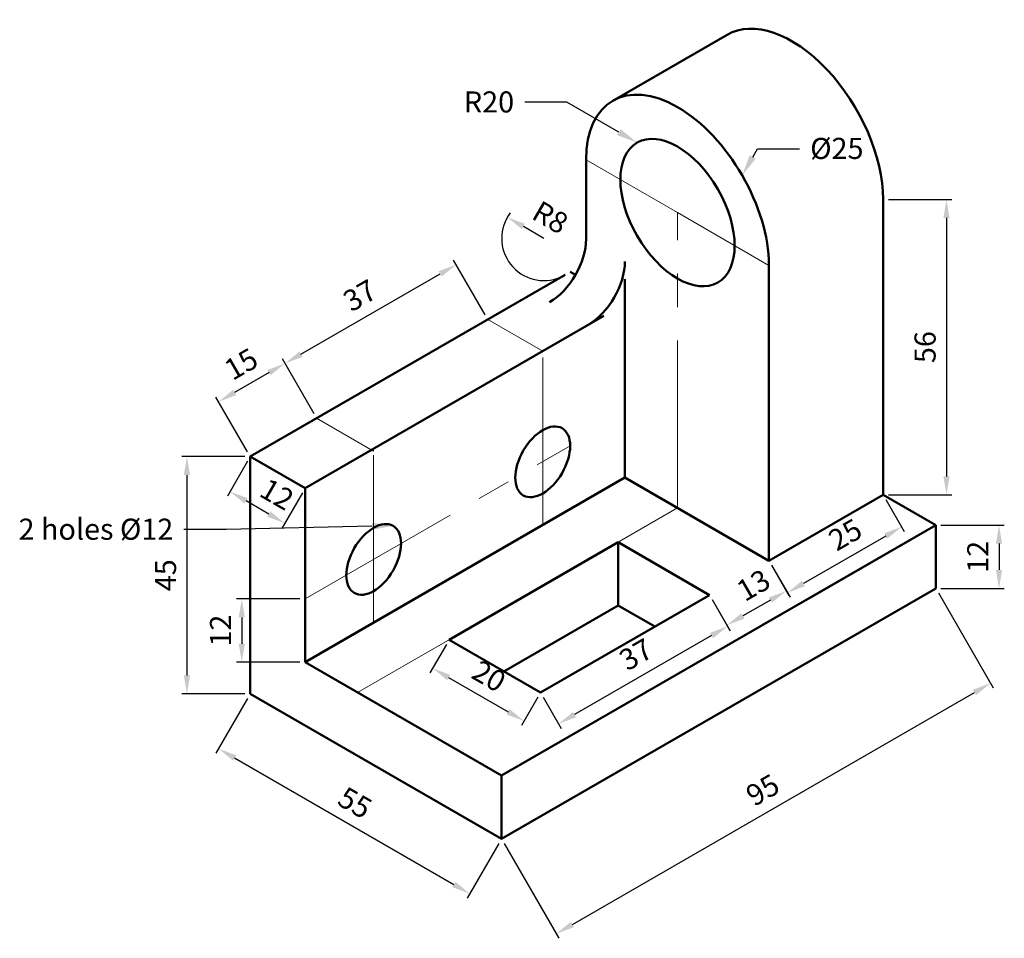
# Model space of a CAD drawing. Units: millimetres. Extents: x 1729 to 1916, y 2075 to 2249.
import ezdxf
from ezdxf import colors
from ezdxf.entities.mleader import LeaderData, LeaderLine
from ezdxf.math import Vec2, Vec3

# ---------------------------------------------------------------- set-up
doc = ezdxf.new("R2010")
doc.units = ezdxf.units.MM
doc.linetypes.add('CENTER', pattern=[50.8, 31.75, -6.35, 6.35, -6.35])
for name, color, linetype, lineweight in [('M-CNTR', 4, 'CENTER', 18), ('M-DIMS', 3, 'Continuous', 25), ('M-OUTL', 7, 'Continuous', 50)]:
    doc.layers.add(name, color=color, linetype=linetype, lineweight=lineweight)
doc.styles.get("Standard").update_dxf_attribs({"font": 'arial.ttf'})
doc.dimstyles.new('AM_ISO$0', dxfattribs={"dimtxt": 4, "dimasz": 3.5, "dimexe": 1, "dimexo": 1, "dimgap": 1.5, "dimtad": 1, "dimdsep": 46, "dimtxsty": 'Standard', "dimcen": 0, "dimclrd": 256, "dimclre": 256, "dimclrt": 2, "dimadec": 0, "dimazin": 2, "dimtp": 0.1, "dimtm": 0.1, "dimtfac": 0.71, "dimtmove": 0, "dimatfit": 3, "dimfxl": 1, "dimlwd": -1, "dimlwe": -1, "dimarcsym": 1})
doc.dimstyles.new('AM_ISO$4', dxfattribs={"dimtxt": 4, "dimasz": 3.5, "dimexe": 1, "dimexo": 1, "dimgap": 1.5, "dimtad": 1, "dimtoh": 1, "dimdsep": 46, "dimtxsty": 'Standard', "dimcen": 0, "dimclrd": 256, "dimclre": 256, "dimclrt": 2, "dimadec": 0, "dimazin": 2, "dimtp": 0.1, "dimtm": 0.1, "dimtfac": 0.71, "dimtofl": 0, "dimtmove": 0, "dimatfit": 0, "dimfxl": 1, "dimlwd": -1, "dimlwe": -1, "dimarcsym": 1})

# ---------------------------------------------------------------- blocks, each defined once
blk = doc.blocks.new('*D3')
at = {"layer": 'Defpoints', "color": 0, "transparency": 16777216}
for p in [(1902.52, 2141.34), (1912.9, 2123.37), (1820.25, 2093.84)]:
    blk.add_point(p, dxfattribs=at)
at = {"layer": 'M-DIMS', "color": 0, "linetype": 'ByBlock', "transparency": 16777216}
for p, q in [((1903.02, 2140.48), (1913.4, 2122.51)), ((1833.66, 2077.62), (1909.87, 2121.62)), ((1820.75, 2092.98), (1831.12, 2075.01))]:
    blk.add_line(p, q, dxfattribs=at)
at = {"layer": 'M-DIMS', "color": 0, "transparency": 16777216}
for points in [[(1909.57, 2122.13), (1910.16, 2121.12), (1912.9, 2123.37)], [(1833.36, 2078.13), (1833.95, 2077.12), (1830.62, 2075.87)]]:
    blk.add_solid(points, dxfattribs=at)
at = {"layer": 'M-DIMS', "color": 0, "transparency": 16777216, "insert": (1869.99, 2102.69), "char_height": 4, "attachment_point": 5, "rotation": 30}
blk.add_mtext('95', dxfattribs=at)
blk = doc.blocks.new('*D4')
at = {"layer": 'Defpoints', "color": 0, "transparency": 16777216}
for p in [(1902.52, 2153.34), (1902.52, 2141.34), (1914.52, 2141.34)]:
    blk.add_point(p, dxfattribs=at)
at = {"layer": 'M-DIMS', "color": 0, "linetype": 'ByBlock', "transparency": 16777216}
for p, q in [((1903.52, 2153.34), (1915.52, 2153.34)), ((1914.52, 2149.84), (1914.52, 2144.84)), ((1903.52, 2141.34), (1915.52, 2141.34))]:
    blk.add_line(p, q, dxfattribs=at)
at = {"layer": 'M-DIMS', "color": 0, "transparency": 16777216}
for points in [[(1913.94, 2149.84), (1915.1, 2149.84), (1914.52, 2153.34)], [(1913.94, 2144.84), (1915.1, 2144.84), (1914.52, 2141.34)]]:
    blk.add_solid(points, dxfattribs=at)
at = {"layer": 'M-DIMS', "color": 0, "transparency": 16777216, "insert": (1911.01, 2147.34), "char_height": 4, "attachment_point": 5, "rotation": 90}
blk.add_mtext('12', dxfattribs=at)
blk = doc.blocks.new('*D5')
at = {"layer": 'Defpoints', "color": 0, "transparency": 16777216}
for p in [(1892.56, 2159.09), (1870.91, 2146.59), (1874.42, 2140.52)]:
    blk.add_point(p, dxfattribs=at)
at = {"layer": 'M-DIMS', "color": 0, "linetype": 'ByBlock', "transparency": 16777216}
for p, q in [((1893.06, 2158.23), (1896.57, 2152.16)), ((1893.04, 2151.27), (1877.45, 2142.27)), ((1871.41, 2145.73), (1874.92, 2139.66))]:
    blk.add_line(p, q, dxfattribs=at)
at = {"layer": 'M-DIMS', "color": 0, "transparency": 16777216}
for points in [[(1892.74, 2151.78), (1893.33, 2150.77), (1896.07, 2153.02)], [(1877.16, 2142.78), (1877.74, 2141.77), (1874.42, 2140.52)]]:
    blk.add_solid(points, dxfattribs=at)
at = {"layer": 'M-DIMS', "color": 0, "transparency": 16777216, "insert": (1885.63, 2151.09), "char_height": 4, "attachment_point": 5, "rotation": 30}
blk.add_mtext('25', dxfattribs=at)
blk = doc.blocks.new('*D6')
at = {"layer": 'Defpoints', "color": 0, "transparency": 16777216}
for p in [(1772.62, 2166.34), (1768.78, 2159.7), (1783.01, 2160.34)]:
    blk.add_point(p, dxfattribs=at)
at = {"layer": 'M-DIMS', "color": 0, "linetype": 'ByBlock', "transparency": 16777216}
for p, q in [((1772.12, 2165.48), (1768.28, 2158.83)), ((1782.51, 2159.48), (1778.67, 2152.83)), ((1776.14, 2155.45), (1771.81, 2157.95))]:
    blk.add_line(p, q, dxfattribs=at)
at = {"layer": 'M-DIMS', "color": 0, "transparency": 16777216}
for points in [[(1772.1, 2158.45), (1771.52, 2157.44), (1768.78, 2159.7)], [(1776.43, 2155.95), (1775.85, 2154.94), (1779.17, 2153.7)]]:
    blk.add_solid(points, dxfattribs=at)
at = {"layer": 'M-DIMS', "color": 0, "transparency": 16777216, "insert": (1777.43, 2158.75), "char_height": 4, "attachment_point": 5, "rotation": 330}
blk.add_mtext('12', dxfattribs=at)
blk = doc.blocks.new('*D7')
at = {"layer": 'Defpoints', "color": 0, "transparency": 16777216}
for p in [(1772.62, 2166.34), (1760.62, 2121.34), (1772.62, 2121.34)]:
    blk.add_point(p, dxfattribs=at)
at = {"layer": 'M-DIMS', "color": 0, "linetype": 'ByBlock', "transparency": 16777216}
for p, q in [((1771.62, 2166.34), (1759.62, 2166.34)), ((1760.62, 2162.84), (1760.62, 2124.84)), ((1771.62, 2121.34), (1759.62, 2121.34))]:
    blk.add_line(p, q, dxfattribs=at)
at = {"layer": 'M-DIMS', "color": 0, "transparency": 16777216}
for points in [[(1760.03, 2162.84), (1761.2, 2162.84), (1760.62, 2166.34)], [(1760.03, 2124.84), (1761.2, 2124.84), (1760.62, 2121.34)]]:
    blk.add_solid(points, dxfattribs=at)
at = {"layer": 'M-DIMS', "color": 0, "transparency": 16777216, "insert": (1757.08, 2143.84), "char_height": 4, "attachment_point": 5, "rotation": 90}
blk.add_mtext('45', dxfattribs=at)
blk = doc.blocks.new('*D8')
at = {"layer": 'Defpoints', "color": 0, "transparency": 16777216}
for p in [(1892.56, 2215.09), (1892.56, 2159.09), (1904.56, 2159.09)]:
    blk.add_point(p, dxfattribs=at)
at = {"layer": 'M-DIMS', "color": 0, "linetype": 'ByBlock', "transparency": 16777216}
for p, q in [((1893.56, 2215.09), (1905.56, 2215.09)), ((1904.56, 2211.59), (1904.56, 2162.59)), ((1893.56, 2159.09), (1905.56, 2159.09))]:
    blk.add_line(p, q, dxfattribs=at)
at = {"layer": 'M-DIMS', "color": 0, "transparency": 16777216}
for points in [[(1903.98, 2211.59), (1905.14, 2211.59), (1904.56, 2215.09)], [(1903.98, 2162.59), (1905.14, 2162.59), (1904.56, 2159.09)]]:
    blk.add_solid(points, dxfattribs=at)
at = {"layer": 'M-DIMS', "color": 0, "transparency": 16777216, "insert": (1901.02, 2187.09), "char_height": 4, "attachment_point": 5, "rotation": 90}
blk.add_mtext('56', dxfattribs=at)
blk = doc.blocks.new('*D9')
at = {"layer": 'Defpoints', "color": 0, "transparency": 16777216}
for p in [(1870.91, 2146.59), (1859.65, 2140.09), (1862.95, 2134.37)]:
    blk.add_point(p, dxfattribs=at)
at = {"layer": 'M-DIMS', "color": 0, "linetype": 'ByBlock', "transparency": 16777216}
for p, q in [((1871.41, 2145.73), (1874.71, 2140.01)), ((1860.15, 2139.23), (1863.45, 2133.51)), ((1871.18, 2139.12), (1865.99, 2136.12))]:
    blk.add_line(p, q, dxfattribs=at)
at = {"layer": 'M-DIMS', "color": 0, "transparency": 16777216}
for points in [[(1870.89, 2139.63), (1871.47, 2138.62), (1874.21, 2140.87)], [(1865.69, 2136.63), (1866.28, 2135.62), (1862.95, 2134.37)]]:
    blk.add_solid(points, dxfattribs=at)
at = {"layer": 'M-DIMS', "color": 0, "transparency": 16777216, "insert": (1868.24, 2141.52), "char_height": 4, "attachment_point": 5, "rotation": 30}
blk.add_mtext('13', dxfattribs=at)
blk = doc.blocks.new('*D10')
at = {"layer": 'Defpoints', "color": 0, "transparency": 16777216}
for p in [(1859.65, 2140.09), (1827.61, 2121.59), (1831.03, 2115.66)]:
    blk.add_point(p, dxfattribs=at)
at = {"layer": 'M-DIMS', "color": 0, "linetype": 'ByBlock', "transparency": 16777216}
for p, q in [((1860.15, 2139.23), (1863.58, 2133.29)), ((1860.05, 2132.41), (1834.07, 2117.41)), ((1828.11, 2120.73), (1831.53, 2114.79))]:
    blk.add_line(p, q, dxfattribs=at)
at = {"layer": 'M-DIMS', "color": 0, "transparency": 16777216}
for points in [[(1859.75, 2132.92), (1860.34, 2131.91), (1863.08, 2134.16)], [(1833.77, 2117.92), (1834.36, 2116.91), (1831.03, 2115.66)]]:
    blk.add_solid(points, dxfattribs=at)
at = {"layer": 'M-DIMS', "color": 0, "transparency": 16777216, "insert": (1845.96, 2128.37), "char_height": 4, "attachment_point": 5, "rotation": 30}
blk.add_mtext('37', dxfattribs=at)
blk = doc.blocks.new('*D11')
at = {"layer": 'Defpoints', "color": 0, "transparency": 16777216}
for p in [(1810.29, 2131.59), (1827.61, 2121.59), (1824.5, 2116.21)]:
    blk.add_point(p, dxfattribs=at)
at = {"layer": 'M-DIMS', "color": 0, "linetype": 'ByBlock', "transparency": 16777216}
for p, q in [((1809.79, 2130.73), (1806.68, 2125.34)), ((1810.21, 2124.46), (1821.47, 2117.96)), ((1827.11, 2120.73), (1824, 2115.34))]:
    blk.add_line(p, q, dxfattribs=at)
at = {"layer": 'M-DIMS', "color": 0, "transparency": 16777216}
for points in [[(1810.5, 2124.96), (1809.92, 2123.95), (1807.18, 2126.21)], [(1821.76, 2118.46), (1821.18, 2117.45), (1824.5, 2116.21)]]:
    blk.add_solid(points, dxfattribs=at)
at = {"layer": 'M-DIMS', "color": 0, "transparency": 16777216, "insert": (1817.61, 2124.27), "char_height": 4, "attachment_point": 5, "rotation": 330}
blk.add_mtext('20', dxfattribs=at)
blk = doc.blocks.new('*D12')
at = {"layer": 'Defpoints', "color": 0, "transparency": 16777216}
for p in [(1772.62, 2121.34), (1820.25, 2093.84), (1814.25, 2083.45)]:
    blk.add_point(p, dxfattribs=at)
at = {"layer": 'M-DIMS', "color": 0, "linetype": 'ByBlock', "transparency": 16777216}
for p, q in [((1772.12, 2120.48), (1766.12, 2110.09)), ((1769.65, 2109.2), (1811.22, 2085.2)), ((1819.75, 2092.98), (1813.75, 2082.59))]:
    blk.add_line(p, q, dxfattribs=at)
at = {"layer": 'M-DIMS', "color": 0, "transparency": 16777216}
for points in [[(1769.94, 2109.71), (1769.36, 2108.7), (1766.62, 2110.95)], [(1811.51, 2085.71), (1810.92, 2084.7), (1814.25, 2083.45)]]:
    blk.add_solid(points, dxfattribs=at)
at = {"layer": 'M-DIMS', "color": 0, "transparency": 16777216, "insert": (1792.2, 2100.26), "char_height": 4, "attachment_point": 5, "rotation": 330}
blk.add_mtext('55', dxfattribs=at)
blk = doc.blocks.new('*D13')
at = {"layer": 'Defpoints', "color": 0, "transparency": 16777216}
for p in [(1811.65, 2202.74), (1817.65, 2192.34), (1785.2, 2173.61)]:
    blk.add_point(p, dxfattribs=at)
at = {"layer": 'M-DIMS', "color": 0, "linetype": 'ByBlock', "transparency": 16777216}
for p, q in [((1817.15, 2193.21), (1811.15, 2203.6)), ((1782.23, 2185.75), (1808.62, 2200.99)), ((1784.7, 2174.47), (1778.7, 2184.87))]:
    blk.add_line(p, q, dxfattribs=at)
at = {"layer": 'M-DIMS', "color": 0, "transparency": 16777216}
for points in [[(1808.33, 2201.49), (1808.91, 2200.48), (1811.65, 2202.74)], [(1781.94, 2186.25), (1782.52, 2185.24), (1779.2, 2184)]]:
    blk.add_solid(points, dxfattribs=at)
at = {"layer": 'M-DIMS', "color": 0, "transparency": 16777216, "insert": (1793.65, 2196.44), "char_height": 4, "attachment_point": 5, "rotation": 30}
blk.add_mtext('37', dxfattribs=at)
blk = doc.blocks.new('*D14')
at = {"layer": 'Defpoints', "color": 0, "transparency": 16777216}
for p in [(1766.62, 2176.74), (1785.2, 2173.61), (1772.62, 2166.34)]:
    blk.add_point(p, dxfattribs=at)
at = {"layer": 'M-DIMS', "color": 0, "linetype": 'ByBlock', "transparency": 16777216}
for p, q in [((1784.7, 2174.47), (1778.7, 2184.87)), ((1776.17, 2182.25), (1769.65, 2178.49)), ((1772.12, 2167.21), (1766.12, 2177.6))]:
    blk.add_line(p, q, dxfattribs=at)
at = {"layer": 'M-DIMS', "color": 0, "transparency": 16777216}
for points in [[(1775.87, 2182.75), (1776.46, 2181.74), (1779.2, 2184)], [(1769.36, 2178.99), (1769.94, 2177.98), (1766.62, 2176.74)]]:
    blk.add_solid(points, dxfattribs=at)
at = {"layer": 'M-DIMS', "color": 0, "transparency": 16777216, "insert": (1771.14, 2183.44), "char_height": 4, "attachment_point": 5, "rotation": 30}
blk.add_mtext('15', dxfattribs=at)
blk = doc.blocks.new('*D15')
at = {"layer": 'Defpoints', "color": 0, "transparency": 16777216}
for p in [(1821.34, 2211.71), (1828.27, 2207.71)]:
    blk.add_point(p, dxfattribs=at)
at = {"layer": 'M-DIMS', "color": 0, "linetype": 'ByBlock', "transparency": 16777216}
blk.add_line((1828.27, 2207.71), (1824.37, 2209.96), dxfattribs=at)
blk.add_arc((1828.27, 2207.71), 8, 142.838, 292.838, dxfattribs=at)
at = {"layer": 'M-DIMS', "color": 0, "transparency": 16777216}
blk.add_solid([(1824.66, 2210.47), (1824.08, 2209.46), (1821.34, 2211.71)], dxfattribs=at)
at = {"layer": 'M-DIMS', "color": 0, "transparency": 16777216, "insert": (1829.24, 2211.24), "char_height": 4, "attachment_point": 5, "rotation": 330}
blk.add_mtext('R8', dxfattribs=at)
blk = doc.blocks.new('*D16')
at = {"layer": 'Defpoints', "color": 0, "transparency": 16777216}
for p in [(1783.01, 2139.34), (1771.01, 2127.34), (1783.01, 2127.34)]:
    blk.add_point(p, dxfattribs=at)
at = {"layer": 'M-DIMS', "color": 0, "linetype": 'ByBlock', "transparency": 16777216}
for p, q in [((1782.01, 2139.34), (1770.01, 2139.34)), ((1771.01, 2135.84), (1771.01, 2130.84)), ((1782.01, 2127.34), (1770.01, 2127.34))]:
    blk.add_line(p, q, dxfattribs=at)
at = {"layer": 'M-DIMS', "color": 0, "transparency": 16777216}
for points in [[(1770.43, 2135.84), (1771.59, 2135.84), (1771.01, 2139.34)], [(1770.43, 2130.84), (1771.59, 2130.84), (1771.01, 2127.34)]]:
    blk.add_solid(points, dxfattribs=at)
at = {"layer": 'M-DIMS', "color": 0, "transparency": 16777216, "insert": (1767.5, 2133.34), "char_height": 4, "attachment_point": 5, "rotation": 90}
blk.add_mtext('12', dxfattribs=at)

msp = doc.modelspace()

# ---------------------------------------------------------------- linework, layer by layer
at = {"layer": 'M-CNTR'}
for p, q in [((1853.589, 2212.594), (1836.269, 2222.594)), ((1853.589, 2156.594), (1853.589, 2212.594)), ((1853.589, 2212.594), (1870.91, 2202.594)), ((1828.042, 2186.344), (1817.649, 2192.344)), ((1828.042, 2153.344), (1828.042, 2186.344)), ((1795.999, 2167.37), (1785.196, 2173.607)), ((1783.008, 2139.344), (1833.238, 2168.344)), ((1795.999, 2134.844), (1795.999, 2167.844)), ((1795.999, 2167.844), (1795.999, 2167.37)), ((1792.968, 2121.594), (1853.589, 2156.594))]:
    msp.add_line(p, q, dxfattribs=at)
at = {"layer": 'M-OUTL'}
for p, q in [((1862.993, 2246.307), (1841.342, 2233.807)), ((1836.269, 2222.594), (1836.269, 2219.713)), ((1836.269, 2219.713), (1836.269, 2207.713)), ((1892.561, 2159.094), (1892.561, 2215.094)), ((1870.91, 2202.594), (1870.91, 2146.594)), ((1772.616, 2166.344), (1832.269, 2200.785)), ((1834.24, 2200.766), (1833.238, 2201.344)), ((1843.63, 2162.344), (1843.63, 2199.963)), ((1783.008, 2160.344), (1839.63, 2193.035)), ((1772.616, 2166.344), (1772.616, 2133.344)), ((1783.008, 2160.344), (1772.616, 2166.344)), ((1783.008, 2127.344), (1843.63, 2162.344)), ((1870.91, 2146.594), (1843.63, 2162.344)), ((1783.008, 2139.344), (1783.008, 2160.344)), ((1870.91, 2146.594), (1892.561, 2159.094)), ((1902.52, 2153.344), (1892.561, 2159.094)), ((1820.248, 2105.844), (1902.52, 2153.344)), ((1902.52, 2153.344), (1880.869, 2140.844)), ((1902.52, 2153.344), (1902.52, 2141.344)), ((1810.288, 2131.594), (1842.331, 2150.094)), ((1842.331, 2150.094), (1859.652, 2140.094)), ((1842.331, 2150.094), (1842.331, 2138.094)), ((1902.52, 2141.344), (1820.248, 2093.844)), ((1880.869, 2140.844), (1869.611, 2134.344)), ((1783.008, 2127.344), (1783.008, 2139.344)), ((1859.652, 2140.094), (1827.609, 2121.594)), ((1820.681, 2125.594), (1842.331, 2138.094)), ((1842.331, 2138.094), (1849.259, 2134.094)), ((1772.616, 2121.344), (1772.616, 2133.344)), ((1827.609, 2121.594), (1810.288, 2131.594)), ((1783.008, 2127.344), (1820.248, 2105.844)), ((1772.616, 2121.344), (1820.248, 2093.844)), ((1820.248, 2093.844), (1820.248, 2105.844))]:
    msp.add_line(p, q, dxfattribs=at)
for centre, major_axis, start_param, end_param in [((1875.24, 2225.094), (12.247, -21.213), 0.7853982, 3.1415927), ((1853.589, 2212.594), (12.247, -21.213), 0.7853982, 3.9269908), ((1829.341, 2203.594), (4.899, 8.485), 3.9269926, 5.4977853), ((1836.702, 2199.344), (4.899, 8.485), 3.9269926, 5.4977853)]:
    msp.add_ellipse(centre, major_axis=major_axis, ratio=0.5773503, start_param=start_param, end_param=end_param, dxfattribs=at)
for centre, major_axis in [((1853.589, 2212.594), (7.655, -13.258)), ((1828.042, 2165.344), (-3.674, -6.364)), ((1795.999, 2146.844), (-3.674, -6.364))]:
    msp.add_ellipse(centre, major_axis=major_axis, ratio=0.5773503, dxfattribs=at)

# ---------------------------------------------------------------- dimensions: what is measured, and where the dimension line sits
at = {"layer": 'M-DIMS'}
dim = msp.add_radius_dim(center=(1828.269, 2207.713), mpoint=(1821.341, 2211.713), dimstyle='AM_ISO$4', override={"dimclrd": 0, "dimclre": 0, "dimclrt": 0}, dxfattribs=at)
dim.commit()
dim.dimension.update_dxf_attribs({"geometry": '*D15', "text_midpoint": (1827.469, 2208.175), "dimtype": 164})
for p1, p2, distance, override, picture, middle in [((1892.561, 2215.094), (1892.561, 2159.094), 12, {"dimpost": '', "dimclrd": 0, "dimclre": 0, "dimclrt": 0}, '*D8', (1901.018, 2187.094)), ((1772.616, 2166.344), (1772.616, 2121.344), -12, {"dimclrd": 0, "dimclre": 0, "dimclrt": 0}, '*D7', (1757.082, 2143.844)), ((1902.52, 2153.344), (1902.52, 2141.344), 12, {"dimclrd": 0, "dimclre": 0, "dimclrt": 0}, '*D4', (1911.012, 2147.344)), ((1820.248, 2093.844), (1902.52, 2141.344), -20.753, {"dimpost": '', "dimclrd": 0, "dimclre": 0, "dimclrt": 0}, '*D3', (1869.989, 2102.689)), ((1810.288, 2131.594), (1827.609, 2121.594), -6.22, {"dimclrd": 0, "dimclre": 0, "dimclrt": 0}, '*D11', (1817.61, 2124.275)), ((1772.616, 2121.344), (1820.248, 2093.844), -12, {"dimpost": '', "dimclrd": 0, "dimclre": 0, "dimclrt": 0}, '*D12', (1792.199, 2100.262))]:
    dim = msp.add_aligned_dim(p1=p1, p2=p2, distance=distance, dimstyle='AM_ISO$0', override=override, dxfattribs=at)
    dim.commit()
    dim.dimension.update_dxf_attribs({"geometry": picture, "text_midpoint": middle})
for p2, distance, text, picture, middle in [((1817.649, 2192.344), 12, '37', '*D13', (1793.651, 2196.437)), ((1772.616, 2166.344), -12, '15', '*D14', (1771.135, 2183.436))]:
    dim = msp.add_aligned_dim(p1=(1785.196, 2173.607), p2=p2, distance=distance, text=text, dimstyle='AM_ISO$0', override={"dimpost": '', "dimclrd": 0, "dimclre": 0, "dimclrt": 0}, dxfattribs=at)
    dim.commit()
    dim.dimension.update_dxf_attribs({"geometry": picture, "text_midpoint": middle})
for base, p1, p2, angle, picture, middle in [((1768.779, 2159.699), (1783.008, 2160.344), (1772.616, 2166.344), 150, '*D6', (1775.677, 2155.716)), ((1874.416, 2140.521), (1892.561, 2159.094), (1870.91, 2146.594), 210, '*D5', (1887.4, 2148.018)), ((1862.955, 2134.373), (1870.91, 2146.594), (1859.652, 2140.094), 210, '*D9', (1870.01, 2138.447)), ((1831.034, 2115.661), (1859.652, 2140.094), (1827.609, 2121.594), 210, '*D10', (1847.736, 2125.304))]:
    dim = msp.add_linear_dim(base=base, p1=p1, p2=p2, angle=angle, dimstyle='AM_ISO$0', override={"dimclrd": 0, "dimclre": 0, "dimclrt": 0}, dxfattribs=at)
    dim.commit()
    dim.dimension.update_dxf_attribs({"geometry": picture, "text_midpoint": middle, "dimtype": 161})
dim = msp.add_linear_dim(base=(1771.008, 2127.344), p1=(1783.008, 2139.344), p2=(1783.008, 2127.344), angle=90, dimstyle='AM_ISO$0', override={"dimpost": '', "dimclrd": 0, "dimclre": 0, "dimclrt": 0}, dxfattribs=at)
dim.commit()
dim.dimension.update_dxf_attribs({"geometry": '*D16', "text_midpoint": (1767.5, 2133.344)})

# ---------------------------------------------------------------- leaders
ml = msp.add_multileader_mtext('Standard', dxfattribs=at)
ml.set_content('{\\C2;R20}', color=256)
ml.set_leader_properties()
ml.build(insert=Vec2(0, 0))
ctx = ml.context
ctx.base_point, ctx.plane_origin = Vec3(1811.078, 2233.538), Vec3(1845.935, 2225.852)
ctx.text_align_type = 2
notes = []
notes.append((ctx, [(0, (1, 1, 0), (1832.622, 2233.538), (-1, 0), 8, [(0, [(1845.935, 2225.852)], 0, [])])]))
ctx.mtext.insert, ctx.mtext.alignment, ctx.mtext.flow_direction = Vec3(1822.622, 2235.572), 3, 5
ml = msp.add_multileader_mtext('Standard', dxfattribs=at)
ml.set_content('{\\C2;%%C25}', color=256)
ml.set_leader_properties()
ml.build(insert=Vec2(0, 0))
ctx = ml.context
ctx.base_point, ctx.plane_origin = Vec3(1876.733, 2224.681), Vec3(1865.837, 2219.665)
notes.append((ctx, [(0, (1, 1, 0), (1868.733, 2224.681), (1, 0), 8, [(0, [(1865.837, 2219.665)], 0, [])])]))
ctx.mtext.insert, ctx.mtext.flow_direction = Vec3(1878.733, 2226.762), 5
ml = msp.add_multileader_mtext('Standard', dxfattribs=at)
ml.set_content('{\\C2;2 holes %%C12}', color=256)
ml.set_leader_properties()
ml.build(insert=Vec2(0, 0))
ctx = ml.context
ctx.base_point, ctx.plane_origin = Vec3(1726.353, 2152.492), Vec3(1799.673, 2153.208)
ctx.text_align_type = 2
notes.append((ctx, [(0, (1, 1, 0), (1768.029, 2152.492), (-1, 0), 8, [(0, [(1799.673, 2153.208)], 0, [])])]))
ctx.mtext.insert, ctx.mtext.alignment, ctx.mtext.flow_direction = Vec3(1758.029, 2154.573), 3, 5
for ctx, leaders in notes:
    for number, flags, end, landing, length, lines in leaders:
        leader = LeaderData()
        leader.index, (leader.has_last_leader_line, leader.has_dogleg_vector, leader.attachment_direction) = number, flags
        leader.last_leader_point, leader.dogleg_vector, leader.dogleg_length = Vec3(end), Vec3(landing), length
        for number, points, colour, breaks in lines:
            line = LeaderLine()
            line.index, line.vertices, line.color, line.breaks = number, Vec3.list(points), colors.encode_raw_color(colour), breaks
            leader.lines.append(line)
        ctx.leaders.append(leader)

doc.saveas('drawing.dxf')
